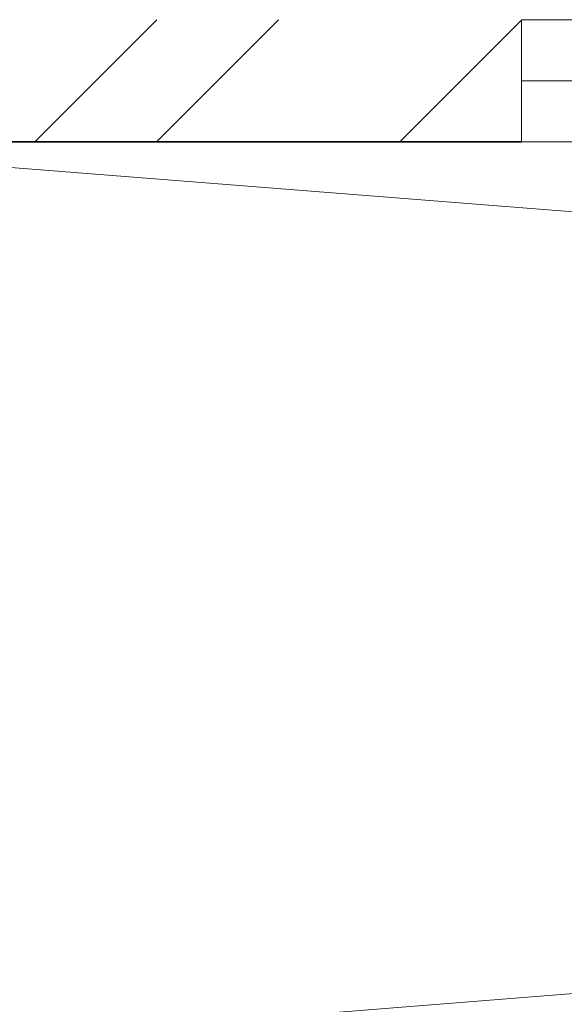
# Model space of a CAD drawing. Units: inches. Extents: x 1885 to 2748, y 783 to 2421.
# Tile 58 of 117: x 2029 to 2049, y 1850 to 1886. Entities that reach past the tile are written whole.
import ezdxf

# ---------------------------------------------------------------- set-up
doc = ezdxf.new("R2010")
doc.units = ezdxf.units.IN
for name, color, linetype, lineweight in [('A-FLOR-OPEN', 8, 'Continuous', 13), ('A-GLAZ', 181, 'Continuous', 18), ('A-WALL', 7, 'Continuous', 35)]:
    doc.layers.add(name, color=color, linetype=linetype, lineweight=lineweight)
doc.layers.add('A-WALL-PATT', color=85, linetype='Continuous', lineweight=13, true_color=0x58ba48)

# ---------------------------------------------------------------- blocks, each defined once
blk = doc.blocks.new('WIN-60')
for p, q in [((0.004, 59.998), (0.004, -0.002)), ((2.254, 59.998), (2.254, -0.002)), ((4.504, -0.002), (4.504, 59.998)), ((2.254, -0.002), (0.004, -0.002)), ((0.004, -0.002), (4.504, -0.002))]:
    blk.add_line(p, q)

msp = doc.modelspace()

# ---------------------------------------------------------------- hatches: boundary and pattern name
at = {"layer": 'A-WALL-PATT'}
h = msp.add_hatch(dxfattribs=at)
h.set_pattern_fill('ANSI32', color=256)
h.paths.add_polyline_path([(2007.772, 2318.006), (1980.774, 2318.006), (1980.774, 2281.215), (1985.274, 2281.215), (1985.274, 2313.506), (2007.772, 2313.506), (2007.772, 2315.756)])
h.paths.add_polyline_path([(2094.324, 2318.006), (2067.772, 2318.006), (2067.772, 2313.506), (2094.324, 2313.506), (2094.324, 2315.756)])
h.paths.add_polyline_path([(2131.367, 2315.756), (2131.367, 2318.006), (2131.189, 2318.006), (2112.609, 2318.006), (2112.609, 2313.506), (2117.274, 2313.506), (2117.274, 2255.201), (2121.774, 2255.201), (2121.774, 2313.506), (2131.367, 2313.506)])
h.paths.add_polyline_path([(2190.512, 2318.006), (2155.367, 2318.006), (2155.367, 2313.506), (2169.774, 2313.506), (2169.774, 2229.506), (2121.774, 2229.506), (2121.774, 2233.451), (2119.524, 2233.451), (2117.274, 2233.451), (2117.274, 2201.101), (2121.774, 2201.101), (2121.774, 2225.006), (2169.774, 2225.006), (2169.774, 2165.006), (2306.274, 2165.006), (2306.274, 2066.006), (2310.774, 2066.006), (2344.274, 2066.006), (2486.274, 2066.006), (2486.274, 1886.006), (2483.02, 1886.006), (2483.02, 1881.506), (2486.274, 1881.506), (2486.274, 1880.678), (2490.774, 1880.678), (2490.774, 2070.506), (2344.274, 2070.506), (2310.774, 2070.506), (2310.774, 2165.006), (2310.774, 2173.636), (2308.524, 2173.636), (2306.274, 2173.636), (2306.274, 2169.506), (2174.274, 2169.506), (2174.274, 2313.506), (2190.512, 2313.506), (2190.512, 2315.756)])
h.paths.add_polyline_path([(1985.274, 2221.215), (1980.774, 2221.215), (1980.774, 2165.006), (1992.774, 2165.006), (1992.774, 2141.927), (1997.274, 2141.927), (1997.274, 2165.006), (2117.274, 2165.006), (2117.274, 2163.126), (2121.774, 2163.126), (2121.774, 2172.734), (2119.524, 2172.734), (2117.274, 2172.734), (2117.274, 2169.506), (1985.274, 2169.506)])
h.paths.add_polyline_path([(1997.274, 2105.927), (1992.774, 2105.927), (1992.774, 2070.506), (2016.774, 2070.506), (2016.774, 2059.123), (2019.024, 2059.123), (2021.274, 2059.123), (2021.274, 2070.506), (2117.274, 2070.506), (2117.274, 2022.506), (2114.423, 2022.506), (2114.423, 2018.006), (2123.627, 2018.006), (2123.627, 2020.256), (2123.627, 2022.506), (2121.774, 2022.506), (2121.774, 2142.587), (2119.524, 2142.587), (2117.274, 2142.587), (2117.274, 2075.006), (1997.274, 2075.006)])
h.paths.add_polyline_path([(2092.029, 2020.256), (2092.029, 2022.506), (2021.274, 2022.506), (2021.274, 2035.123), (2016.774, 2035.123), (2016.774, 2018.006), (2016.774, 1978.784), (2021.274, 1978.784), (2021.274, 2018.006), (2092.029, 2018.006)])
h.paths.add_polyline_path([(2260.938, 2022.506), (2153.105, 2022.506), (2153.105, 2020.256), (2153.105, 2018.006), (2155.274, 2018.006), (2155.274, 1886.006), (2107.629, 1886.006), (2107.629, 1881.506), (2182.911, 1881.506), (2182.911, 1883.756), (2182.911, 1886.006), (2159.774, 1886.006), (2159.774, 2018.006), (2260.938, 2018.006), (2260.938, 2020.256)])
h.paths.add_polyline_path([(2047.629, 1883.756), (2047.629, 1886.006), (2021.274, 1886.006), (2021.274, 1918.784), (2019.024, 1918.784), (2016.774, 1918.784), (2016.774, 1881.506), (2047.629, 1881.506)])
h.paths.add_polyline_path([(2306.361, 1883.756), (2306.361, 1886.006), (2296.274, 1886.006), (2296.274, 1982.006), (2316.535, 1982.006), (2316.535, 1984.256), (2316.535, 1986.506), (2296.274, 1986.506), (2296.274, 2022.506), (2289.276, 2022.506), (2289.276, 2018.006), (2291.774, 2018.006), (2291.774, 1886.006), (2242.911, 1886.006), (2242.911, 1881.506), (2306.361, 1881.506)], flags=17)
h.paths.add_polyline_path([(1985.274, 1843.006), (2021.6, 1843.006), (2021.534, 1845.441), (2021.477, 1847.506), (1980.774, 1847.506), (1980.774, 1809.446), (1985.274, 1809.446)])
h.paths.add_polyline_path([(2131.482, 1845.256), (2131.482, 1847.506), (2081.534, 1847.506), (2081.534, 1843.006), (2117.274, 1843.006), (2117.274, 1784.147), (2119.524, 1784.147), (2121.774, 1784.147), (2121.774, 1843.006), (2131.482, 1843.006)])
h.paths.add_polyline_path([(2203.886, 1847.506), (2155.482, 1847.506), (2155.482, 1843.006), (2169.774, 1843.006), (2169.774, 1759.006), (2121.774, 1759.006), (2121.774, 1761.457), (2117.274, 1761.457), (2117.274, 1730.429), (2121.774, 1730.429), (2121.774, 1754.506), (2177.421, 1754.506), (2177.421, 1756.756), (2177.421, 1759.006), (2174.274, 1759.006), (2174.274, 1843.006), (2203.886, 1843.006)])
h.paths.add_polyline_path([(2335.554, 1845.256), (2335.554, 1847.506), (2239.886, 1847.506), (2239.886, 1843.006), (2306.274, 1843.006), (2306.274, 1759.006), (2199.486, 1759.006), (2199.486, 1754.506), (2310.774, 1754.506), (2310.774, 1843.006), (2335.554, 1843.006)])
h.paths.add_polyline_path([(2348.774, 2022.506), (2344.274, 2022.506), (2344.274, 1986.506), (2341.681, 1986.506), (2341.681, 1982.006), (2344.274, 1982.006), (2344.274, 1886.006), (2330.361, 1886.006), (2330.361, 1881.506), (2361.627, 1881.506), (2361.627, 1883.756), (2361.627, 1886.006), (2348.774, 1886.006)], flags=17)
h.paths.add_polyline_path([(2283.251, 2315.756), (2283.251, 2318.006), (2238.512, 2318.006), (2238.512, 2313.506), (2283.251, 2313.506)], flags=17)
h.paths.add_polyline_path([(2363.274, 2348.006), (2388.677, 2348.006), (2388.677, 2350.256), (2388.677, 2352.506), (2358.774, 2352.506), (2358.774, 2348.006), (2358.774, 2318.006), (2344.481, 2318.006), (2344.481, 2313.506), (2358.774, 2313.506), (2358.774, 2229.506), (2310.774, 2229.506), (2310.774, 2231.952), (2306.274, 2231.952), (2306.274, 2205.611), (2310.774, 2205.611), (2310.774, 2225.006), (2358.774, 2225.006), (2358.774, 2211.506), (2452.329, 2211.506), (2452.329, 2213.756), (2452.329, 2216.006), (2363.274, 2216.006), (2363.274, 2318.006)])
h.paths.add_polyline_path([(2310.774, 2313.506), (2320.481, 2313.506), (2320.481, 2315.756), (2320.481, 2318.006), (2302.728, 2318.006), (2302.728, 2313.506), (2306.274, 2313.506), (2306.274, 2251.076), (2310.774, 2251.076)], flags=17)
h.paths.add_polyline_path([(2490.774, 2352.506), (2486.274, 2352.506), (2448.677, 2352.506), (2448.677, 2348.006), (2486.274, 2348.006), (2486.274, 2318.006), (2486.274, 2216.006), (2481.78, 2216.006), (2481.78, 2211.506), (2486.274, 2211.506), (2486.274, 2165.006), (2493.289, 2165.006), (2493.289, 2167.256), (2493.289, 2169.506), (2490.774, 2169.506), (2490.774, 2313.506), (2494.429, 2313.506), (2494.429, 2318.006), (2490.774, 2318.006)])
h.paths.add_polyline_path([(2534.653, 2318.006), (2515.691, 2318.006), (2515.691, 2313.506), (2534.653, 2313.506), (2534.653, 2315.756)])
h.paths.add_polyline_path([(2618.274, 2318.006), (2594.653, 2318.006), (2594.653, 2313.506), (2613.774, 2313.506), (2613.774, 2281.706), (2618.274, 2281.706)])
h.paths.add_polyline_path([(2618.274, 2221.706), (2613.774, 2221.706), (2613.774, 2169.506), (2554.019, 2169.506), (2554.019, 2165.006), (2613.774, 2165.006), (2613.774, 2152.878), (2618.274, 2152.878)])
h.paths.add_polyline_path([(2618.274, 2128.878), (2616.024, 2128.878), (2613.774, 2128.878), (2613.774, 2117.006), (2529.774, 2117.006), (2529.774, 2165.006), (2532.848, 2165.006), (2532.848, 2169.506), (2522.867, 2169.506), (2522.867, 2165.006), (2525.274, 2165.006), (2525.274, 2117.006), (2525.274, 2112.506), (2525.274, 2108.576), (2529.774, 2108.576), (2529.774, 2112.506), (2613.774, 2112.506), (2613.774, 2080.19), (2618.274, 2080.19)])
h.paths.add_polyline_path([(2618.274, 2044.19), (2616.024, 2044.19), (2613.774, 2044.19), (2613.774, 2015.506), (2529.774, 2015.506), (2529.774, 2088.582), (2527.524, 2088.582), (2525.274, 2088.582), (2525.274, 2011.006), (2613.774, 2011.006), (2613.774, 1956.755), (2618.274, 1956.755)])
h.paths.add_polyline_path([(2618.274, 1881.506), (2618.274, 1896.755), (2613.774, 1896.755), (2613.774, 1881.506), (2613.774, 1847.506), (2592.715, 1847.506), (2592.715, 1843.006), (2613.774, 1843.006), (2613.774, 1765.006), (2613.774, 1760.506), (2609.621, 1760.506), (2609.621, 1756.006), (2613.774, 1756.006), (2613.774, 1660.006), (2608.544, 1660.006), (2608.544, 1655.506), (2613.774, 1655.506), (2613.774, 1508.158), (2618.274, 1508.158)])
h.paths.add_polyline_path([(2565.774, 1843.006), (2568.997, 1843.006), (2568.997, 1847.506), (2490.774, 1847.506), (2490.774, 1849.7), (2488.524, 1849.7), (2486.274, 1849.7), (2486.274, 1847.506), (2477.274, 1847.506), (2477.274, 1838.506), (2477.274, 1821.493), (2486.274, 1821.493), (2486.274, 1838.506), (2561.274, 1838.506), (2561.274, 1765.006), (2486.274, 1765.006), (2486.274, 1786.157), (2477.274, 1786.157), (2477.274, 1765.006), (2477.274, 1756.006), (2486.274, 1756.006), (2565.774, 1756.006), (2585.621, 1756.006), (2585.621, 1758.256), (2585.621, 1760.506), (2565.774, 1760.506), (2565.774, 1765.006)])
h.paths.add_polyline_path([(2486.274, 1651.006), (2561.274, 1651.006), (2561.274, 1567.006), (2486.274, 1567.006), (2486.274, 1591.321), (2477.274, 1591.321), (2477.274, 1567.006), (2477.274, 1558.006), (2477.274, 1555.439), (2481.774, 1555.439), (2481.774, 1558.006), (2568.653, 1558.006), (2568.653, 1560.256), (2568.653, 1562.506), (2565.774, 1562.506), (2565.774, 1655.506), (2584.544, 1655.506), (2584.544, 1657.756), (2584.544, 1660.006), (2565.774, 1660.006), (2486.274, 1660.006), (2477.274, 1660.006), (2477.274, 1651.006), (2477.274, 1632.989), (2486.274, 1632.989)])
h.paths.add_polyline_path([(2449.967, 1883.756), (2449.967, 1886.006), (2421.627, 1886.006), (2421.627, 1881.506), (2449.967, 1881.506)], flags=17)
h.paths.add_polyline_path([(2447.274, 1847.506), (2395.554, 1847.506), (2395.554, 1843.006), (2442.774, 1843.006), (2442.774, 1809.27), (2447.274, 1809.27)])
h.paths.add_polyline_path([(1985.274, 1749.446), (1980.774, 1749.446), (1980.774, 1694.504), (1985.274, 1694.504), (1985.274, 1694.506), (1986.897, 1694.506), (1986.897, 1697.78), (1986.897, 1699.006), (1985.274, 1699.006)])
h.paths.add_polyline_path([(2152.774, 1699.006), (2121.774, 1699.006), (2121.774, 1703.668), (2119.524, 1703.668), (2117.274, 1703.668), (2117.274, 1699.006), (2009.219, 1699.006), (2009.219, 1694.506), (2148.274, 1694.506), (2148.274, 1692.631), (2152.774, 1692.631)])
h.paths.add_polyline_path([(2016.274, 1694.506), (2011.774, 1694.506), (2011.774, 1558.006), (2040.806, 1558.006), (2040.806, 1560.256), (2040.806, 1562.506), (2016.274, 1562.506)])
h.paths.add_polyline_path([(2152.774, 1663.017), (2150.524, 1663.017), (2148.274, 1663.017), (2148.274, 1562.506), (2100.806, 1562.506), (2100.806, 1558.006), (2165.119, 1558.006), (2165.119, 1560.256), (2165.119, 1562.506), (2152.774, 1562.506), (2152.774, 1610.506), (2224.774, 1610.506), (2224.774, 1607.99), (2229.274, 1607.99), (2229.274, 1615.006), (2152.774, 1615.006)])
h.paths.add_polyline_path([(2238.613, 1560.256), (2238.613, 1562.506), (2229.274, 1562.506), (2229.274, 1588.756), (2227.024, 1588.763), (2224.774, 1588.771), (2224.774, 1562.506), (2189.119, 1562.506), (2189.119, 1558.006), (2238.613, 1558.006)])
h.paths.add_polyline_path([(2336.024, 1560.256), (2336.024, 1562.506), (2310.774, 1562.506), (2310.774, 1656.347), (2308.524, 1656.347), (2306.274, 1656.347), (2306.274, 1562.506), (2286.613, 1562.506), (2286.613, 1558.006), (2336.024, 1558.006)])
h.paths.add_polyline_path([(2447.274, 1690.968), (2445.024, 1690.968), (2442.774, 1690.968), (2442.774, 1687.006), (2306.274, 1687.006), (2306.274, 1680.75), (2310.774, 1680.75), (2310.774, 1682.506), (2442.774, 1682.506), (2442.774, 1562.506), (2396.024, 1562.506), (2396.024, 1558.006), (2447.274, 1558.006)])
h.paths.add_polyline_path([(2447.274, 1749.27), (2445.024, 1749.27), (2442.774, 1749.27), (2442.774, 1717.232), (2447.274, 1717.232)])
h.paths.add_polyline_path([(2044.674, 1521.756), (2044.674, 1524.006), (2007.274, 1524.006), (2007.274, 1503.49), (2009.524, 1503.49), (2011.774, 1503.49), (2011.774, 1519.506), (2044.674, 1519.506)])
h.paths.add_polyline_path([(2177.969, 1521.756), (2177.969, 1524.006), (2104.674, 1524.006), (2104.674, 1519.506), (2145.774, 1519.506), (2145.774, 1387.506), (2143.37, 1387.506), (2143.37, 1383.006), (2251.585, 1383.006), (2251.585, 1385.256), (2251.585, 1387.506), (2150.274, 1387.506), (2150.274, 1519.506), (2177.969, 1519.506)])
h.paths.add_polyline_path([(2298.704, 1524.006), (2237.969, 1524.006), (2237.969, 1519.506), (2282.274, 1519.506), (2282.274, 1387.506), (2279.683, 1387.506), (2279.683, 1383.006), (2286.774, 1383.006), (2286.774, 1419.006), (2312.451, 1419.006), (2312.451, 1421.256), (2312.451, 1423.506), (2286.774, 1423.506), (2286.774, 1519.506), (2298.704, 1519.506), (2298.704, 1521.722)], flags=17)
h.paths.add_polyline_path([(2361.897, 1521.756), (2361.897, 1524.006), (2322.704, 1524.006), (2322.704, 1519.506), (2334.774, 1519.506), (2334.774, 1423.506), (2331.93, 1423.506), (2331.93, 1419.006), (2334.774, 1419.006), (2334.774, 1387.506), (2334.774, 1383.228), (2339.274, 1383.228), (2339.274, 1387.506), (2339.274, 1519.506), (2361.897, 1519.506)], flags=17)
h.paths.add_polyline_path([(2447.274, 1521.756), (2447.274, 1524.006), (2421.897, 1524.006), (2421.897, 1519.506), (2447.274, 1519.506)], flags=17)
h.paths.add_polyline_path([(2481.774, 1529.6), (2479.524, 1529.6), (2477.274, 1529.6), (2477.274, 1524.006), (2474.489, 1524.006), (2474.489, 1519.506), (2477.274, 1519.506), (2477.274, 1334.506), (2296.774, 1334.506), (2296.774, 1240.506), (2160.274, 1240.506), (2160.274, 1180.506), (2112.274, 1180.506), (2112.274, 1207.692), (2110.024, 1207.692), (2107.774, 1207.692), (2107.774, 1171.609), (2112.274, 1171.609), (2112.274, 1176.006), (2160.274, 1176.006), (2160.274, 1092.006), (2144.221, 1092.006), (2144.221, 1087.506), (2189.497, 1087.506), (2189.497, 1089.756), (2189.497, 1092.006), (2164.774, 1092.006), (2164.774, 1236.006), (2296.774, 1236.006), (2296.774, 1231.912), (2301.274, 1231.912), (2301.274, 1330.006), (2481.774, 1330.006), (2481.774, 1387.506)])
h.paths.add_polyline_path([(2618.274, 1448.158), (2613.774, 1448.158), (2613.774, 1382.506), (2529.774, 1382.506), (2525.274, 1382.506), (2525.274, 1307.062), (2529.774, 1307.062), (2529.774, 1378.006), (2613.774, 1378.006), (2613.774, 1354.988), (2618.274, 1354.988)])
h.paths.add_polyline_path([(2618.274, 1318.988), (2613.774, 1318.988), (2613.774, 1281.006), (2529.774, 1281.006), (2529.774, 1283.786), (2527.524, 1283.786), (2525.274, 1283.786), (2525.274, 1228.506), (2516.794, 1228.506), (2516.794, 1224.006), (2533.484, 1224.006), (2533.484, 1226.256), (2533.484, 1228.506), (2529.774, 1228.506), (2529.774, 1276.506), (2613.774, 1276.506), (2613.774, 1266.02), (2618.274, 1266.02)])
h.paths.add_polyline_path([(2618.274, 1134.964), (2613.774, 1134.964), (2613.774, 1092.006), (2594.545, 1092.006), (2594.545, 1087.506), (2618.274, 1087.506)])
h.paths.add_polyline_path([(2534.545, 1092.006), (2509.765, 1092.006), (2509.765, 1087.506), (2534.545, 1087.506), (2534.545, 1089.756)])
h.paths.add_polyline_path([(2481.274, 1224.006), (2484.117, 1224.006), (2484.117, 1226.256), (2484.117, 1228.506), (2476.774, 1228.506), (2476.774, 1198.506), (2471.61, 1198.506), (2471.61, 1194.006), (2476.774, 1194.006), (2476.774, 1062.006), (2436.894, 1062.006), (2436.894, 1057.506), (2476.774, 1057.506), (2481.274, 1057.506), (2481.274, 1062.006), (2481.274, 1087.506), (2485.354, 1087.506), (2485.354, 1089.756), (2485.354, 1092.006), (2481.274, 1092.006), (2481.274, 1117.506)])
h.paths.add_polyline_path([(2439.898, 1198.506), (2349.274, 1198.506), (2349.274, 1194.006), (2349.274, 1180.506), (2301.274, 1180.506), (2301.274, 1201.896), (2299.024, 1201.896), (2296.774, 1201.896), (2296.774, 1172.335), (2299.024, 1172.335), (2301.274, 1172.335), (2301.274, 1176.006), (2349.274, 1176.006), (2349.274, 1092.006), (2334.452, 1092.006), (2334.452, 1087.506), (2349.274, 1087.506), (2349.274, 1057.506), (2353.774, 1057.506), (2376.894, 1057.506), (2376.894, 1059.756), (2376.894, 1062.006), (2353.774, 1062.006), (2353.774, 1087.506), (2353.774, 1180.506), (2353.774, 1194.006), (2439.898, 1194.006), (2439.898, 1196.256)])
h.paths.add_polyline_path([(2270.596, 1089.756), (2270.596, 1092.006), (2249.497, 1092.006), (2249.497, 1087.506), (2270.596, 1087.506)], flags=17)
h.paths.add_polyline_path([(2310.452, 1092.006), (2301.274, 1092.006), (2301.274, 1153.292), (2296.774, 1153.292), (2296.774, 1092.006), (2293.786, 1092.006), (2293.786, 1087.506), (2310.452, 1087.506), (2310.452, 1089.756)], flags=17)
h.paths.add_polyline_path([(2112.274, 1150.328), (2110.024, 1150.328), (2107.774, 1150.328), (2107.774, 1092.006), (2104.465, 1092.006), (2104.465, 1087.506), (2120.221, 1087.506), (2120.221, 1089.756), (2120.221, 1092.006), (2112.274, 1092.006)])
h.paths.add_polyline_path([(2082.172, 1092.006), (2058.144, 1092.006), (2058.144, 1087.506), (2082.172, 1087.506), (2082.172, 1089.756)])
h.paths.add_polyline_path([(1975.774, 1145.638), (1971.274, 1145.638), (1971.274, 1087.506), (1980.774, 1087.506), (1998.144, 1087.506), (1998.144, 1089.756), (1998.144, 1092.006), (1985.274, 1092.006), (1975.774, 1092.006)])
h.paths.add_polyline_path([(2112.274, 1244.385), (2110.024, 1244.385), (2107.774, 1244.385), (2107.774, 1240.506), (1992.274, 1240.506), (1992.274, 1271.008), (1987.774, 1271.008), (1987.774, 1240.506), (1980.774, 1240.506), (1975.774, 1240.506), (1971.274, 1240.506), (1971.274, 1205.638), (1975.774, 1205.638), (1975.774, 1236.006), (2107.774, 1236.006), (2107.774, 1233.444), (2112.274, 1233.444), (2112.274, 1236.006)])
h.paths.add_polyline_path([(2112.274, 1383.006), (2114.783, 1383.006), (2114.783, 1385.256), (2114.783, 1387.506), (2102.476, 1387.506), (2102.476, 1383.006), (2107.774, 1383.006), (2107.774, 1335.006), (2011.774, 1335.006), (2011.774, 1349.939), (2007.274, 1349.939), (2007.274, 1335.006), (1987.774, 1335.006), (1987.774, 1330.506), (1987.774, 1307.008), (1992.274, 1307.008), (1992.274, 1330.506), (2007.274, 1330.506), (2107.774, 1330.506), (2107.774, 1264.711), (2112.274, 1264.711)])
h.paths.add_polyline_path([(2077.857, 1387.506), (2011.774, 1387.506), (2011.774, 1390.036), (2009.524, 1390.036), (2007.274, 1390.036), (2007.274, 1373.939), (2011.774, 1373.939), (2011.774, 1383.006), (2077.857, 1383.006)])
h.paths.add_polyline_path([(2011.774, 1443.49), (2007.274, 1443.49), (2007.274, 1410.248), (2011.774, 1410.248)])

# ---------------------------------------------------------------- linework, layer by layer
at = {"layer": 'A-FLOR-OPEN'}
for p, q in [((2016.774, 1847.506), (2447.274, 1881.506)), ((2447.274, 1847.506), (2016.774, 1881.506))]:
    msp.add_line(p, q, dxfattribs=at)
at = {"layer": 'A-WALL'}
msp.add_line((2016.774, 1881.506), (2047.629, 1881.506), dxfattribs=at)
msp.add_line((2016.774, 1881.506), (2047.629, 1881.506), dxfattribs=at)

# ---------------------------------------------------------------- block references
at = {"layer": 'A-GLAZ', "extrusion": (0, 0, -1), "zscale": -1, "rotation": 90}
msp.add_blockref('WIN-60', (-2047.632, 1881.502), dxfattribs=at)

doc.saveas('drawing.dxf')
